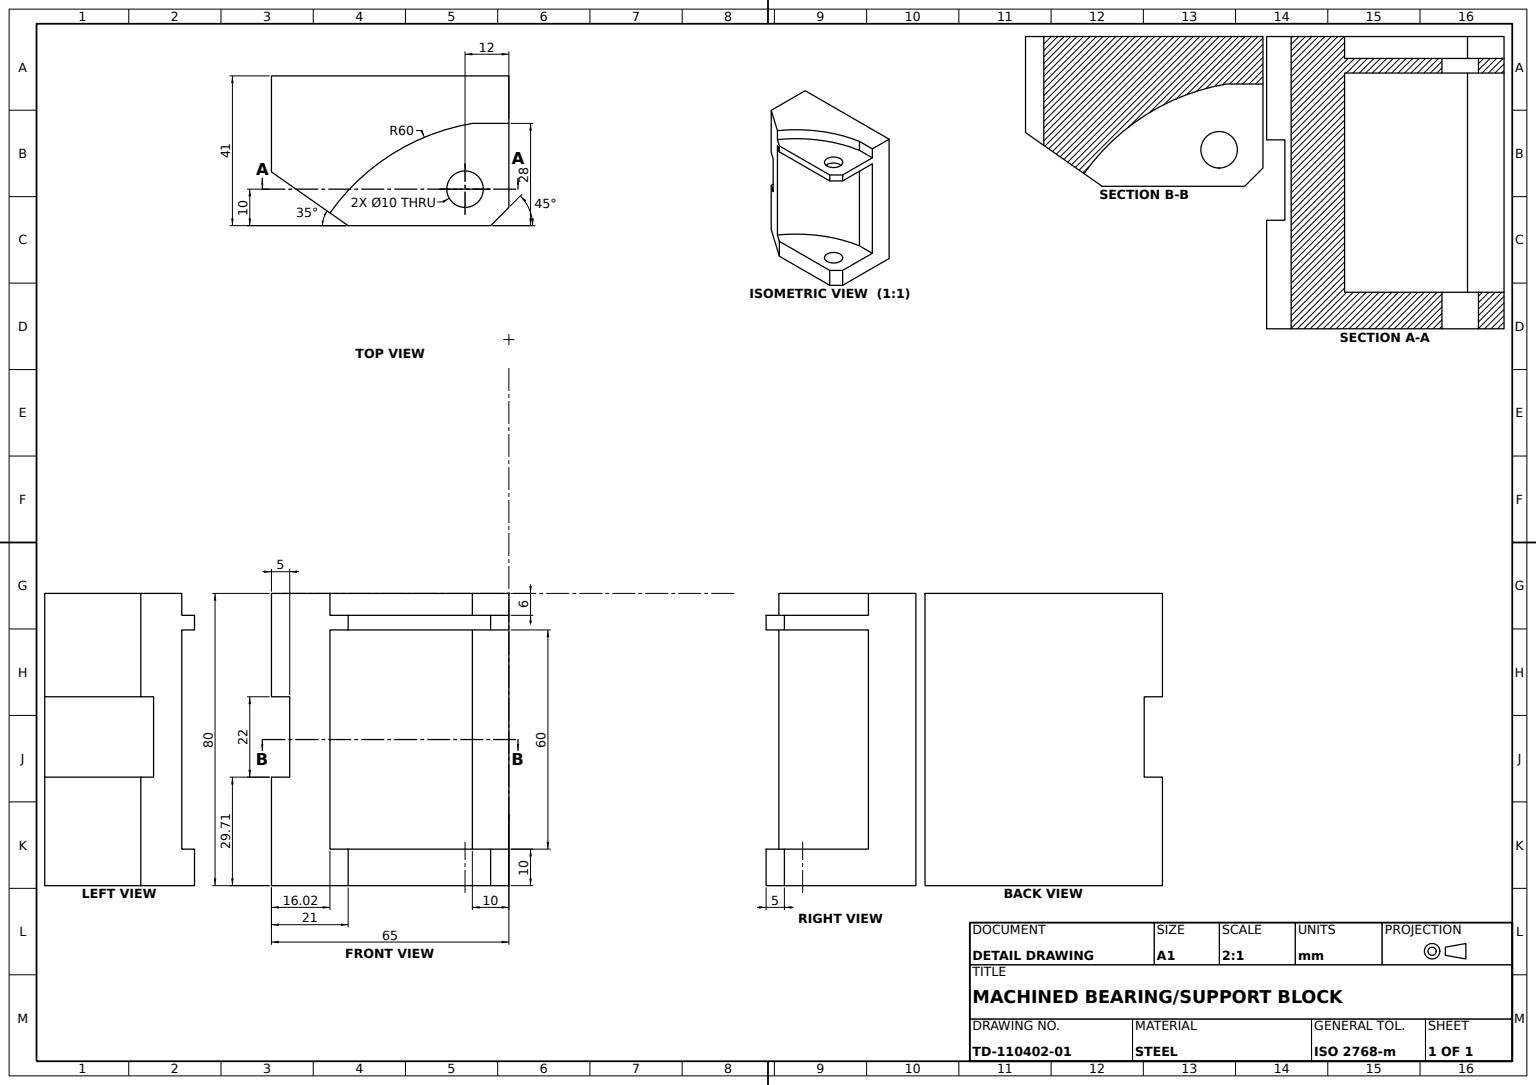
SolidWorks part; units mm, degrees
material "Plain Carbon Steel"
ref_plane "Front Plane" through (0, 0, 0) normal (0, 0, 1) x (1, 0, 0)
ref_plane "Top Plane" through (0, 0, 0) normal (0, 1, 0) x (1, 0, 0)
ref_plane "Right Plane" through (0, 0, 0) normal (1, 0, 0) x (0, 0, -1)
sketch "Base Block Profile Sketch" plane through (0, 0, 0) normal (0, 1, 0) x (1, 0, 0)
  line L0 (11.5, 20.5) -> (32.5, 5.7956)
  line L1 (-27.5, 20.5) -> (11.5, 20.5)
  line L2 (-32.5, 15.5) -> (-32.5, -20.5)
  line L3 (-32.5, -20.5) -> (32.5, -20.5)
  line L4 (32.5, 5.7956) -> (32.5, -20.5)
  line L5 (-32.5, 15.5) -> (-27.5, 20.5)
  point P0 (0, 0)
  point P2 (-32.5, 20.5)
  point P4 (32.5, 20.5)
  dimension "D1" = 65
  dimension "D2" = 41
  dimension "D3" = 21
  dimension "D4" = 35
  dimension "D5" = 5
  dimension "D6" = 45
  dimension "D7" = 32.5
  dimension "D8" = 20.5
extrude "Base Block" add sketch "Base Block Profile Sketch" along normal mid plane 80
sketch "Side Slot Sketch" plane through (0, 0, 0) normal (0, 0, 1) x (1, 0, 0)
  line L0 (32.5, 40) -> (32.5, -40) construction
  line L1 (27.5, -10.2925) -> (32.5, -10.2925)
  line L2 (27.5, -10.2925) -> (27.5, 11.7075)
  line L3 (27.5, 11.7075) -> (32.5, 11.7075)
  line L4 (32.5, -10.2925) -> (32.5, 11.7075)
  line L5 (27.5, -10.2925) -> (32.5, 11.7075) construction
  line L6 (27.5, 11.7075) -> (32.5, -10.2925) construction
  point P0 (30, 0.7075)
  dimension "D1" = 5
  dimension "D2" = 22
  dimension "D3" = 0.7075
extrude "Side Slot" cut sketch "Side Slot Sketch" along normal through all both and the other way through all
sketch "Top Step Pocket Sketch" plane through (0, 40, 0) normal (0, 1, 0) x (1, 0, 0)
  line L0 (11.5, 20.5) -> (-27.5, 20.5) construction
  line L1 (32.5, 5.7956) -> (11.5, 20.5) construction
  line L2 (-27.5, 20.5) -> (-32.5, 15.5) construction
  line L3 (-32.5, 15.5) -> (-32.5, -20.5) construction
  line L4 (16.4833, 17.0106) -> (11.5, 20.5)
  line L5 (11.5, 20.5) -> (-27.5, 20.5)
  line L6 (-27.5, 20.5) -> (-32.5, 15.5)
  line L7 (-32.5, 15.5) -> (-32.5, -7.5)
  line L8 (-32.5, -7.5) -> (-22.5, -7.5)
  arc A0 (-22.5, -7.5) -> (16.4833, 17.0106) centre (-32.5, 51.6608) ccw
  dimension "D4" = 60
  dimension "D1" = 0
  dimension "D2" = 28
  dimension "D3" = 10
extrude "Top Step Pocket" cut sketch "Top Step Pocket Sketch" against normal blind 6
sketch "Arc Relief Sketch" plane through (0, 0, 0) normal (0, 1, 0) x (1, 0, 0)
  line L0 (-27.5, 20.5) -> (-32.5, 15.5) construction
  line L1 (-32.5, 15.5) -> (-32.5, -7.5) construction
  line L2 (-32.5, -7.5) -> (-22.5, -7.5) construction
  line L3 (11.5, 20.5) -> (-27.5, 20.5) construction
  line L4 (16.4833, 17.0106) -> (11.5, 20.5) construction
  line L5 (-27.5, 20.5) -> (-32.5, 15.5)
  line L6 (-32.5, 15.5) -> (-32.5, -7.5)
  line L7 (-32.5, -7.5) -> (-22.5, -7.5)
  line L8 (11.5, 20.5) -> (-27.5, 20.5)
  line L9 (16.4833, 17.0106) -> (11.5, 20.5)
  arc A0 (-22.5, -7.5) -> (16.4833, 17.0106) centre (-32.5, 51.6608) ccw construction
  arc A1 (-22.5, -7.5) -> (16.4833, 17.0106) centre (-32.5, 51.6608) ccw
extrude "Arc Relief Cut" cut sketch "Arc Relief Sketch" against normal mid plane 60
sketch "Through Hole Sketch" plane through (0, 34, 0) normal (0, 1, 0) x (1, 0, 0)
  line L0 (-32.5, 15.5) -> (-32.5, -7.5) construction
  line L1 (11.5, 20.5) -> (-27.5, 20.5) construction
  circle A0 centre (-20.5, 10.5) radius 5
  dimension "D1" = 10
  dimension "D2" = 12
  dimension "D3" = 10
extrude "Through Hole" cut sketch "Through Hole Sketch" against normal blind 110
